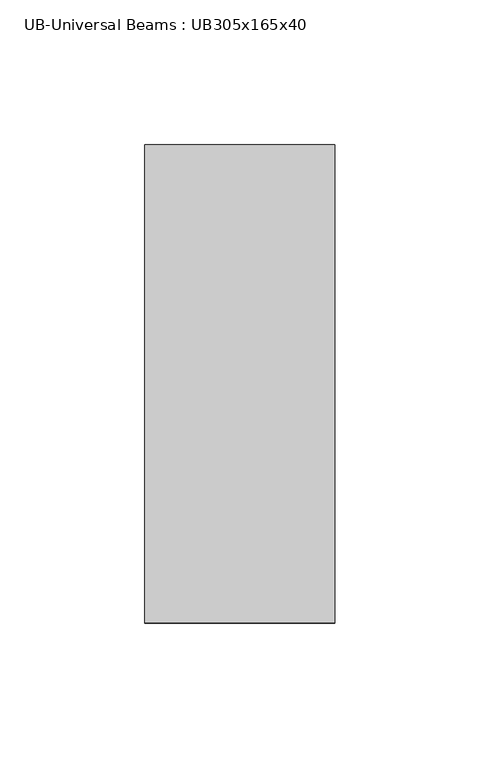
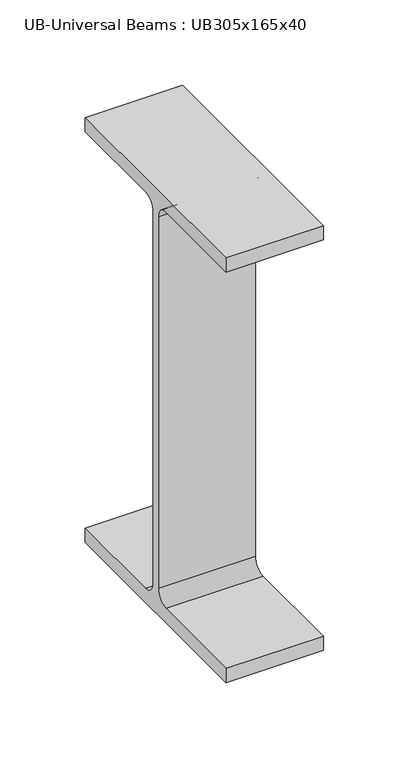
"""IFC4 building model written with IfcOpenShell, lengths in millimetres: beam geometry, UB-Universal Beams : UB305x165x40."""

from ifc_helpers import new_model, si_unit, point, frame, frame_2d, origin, place, context, project, spatial, polyline, circle_curve, trimmed, segment, composite_curve, outline, extrude, source, transform, mapped, element, save


def ub_universal_beams_ub305x165x40_454c3f6d(model_context):
    return source(origin(), model_context, "Body", "SweptSolid", [
        extrude(outline(composite_curve([segment(polyline([(82.5, -141.5), (82.5, -151.7), (-82.5, -151.7), (-82.5, -141.5), (-11.9, -141.5)]), True, "CONTINUOUS"), segment(trimmed(circle_curve(frame_2d((-11.9, -132.6)), 8.9), [point((-11.9, -141.5))], [point((-3.0, -132.6))], True, "CARTESIAN"), True, "CONTINUOUS"), segment(polyline([(-3.0, -132.6), (-3.0, 132.6)]), True, "CONTINUOUS"), segment(trimmed(circle_curve(frame_2d((-11.9, 132.6)), 8.9), [point((-3.0, 132.6))], [point((-11.9, 141.5))], True, "CARTESIAN"), True, "CONTINUOUS"), segment(polyline([(-11.9, 141.5), (-82.5, 141.5), (-82.5, 151.7), (82.5, 151.7), (82.5, 141.5), (11.9, 141.5)]), True, "CONTINUOUS"), segment(trimmed(circle_curve(frame_2d((11.9, 132.6)), 8.9), [point((11.9, 141.5))], [point((3.0, 132.6))], True, "CARTESIAN"), True, "CONTINUOUS"), segment(polyline([(3.0, 132.6), (3.0, -132.6)]), True, "CONTINUOUS"), segment(trimmed(circle_curve(frame_2d((11.9, -132.6)), 8.9), [point((3.0, -132.6))], [point((11.9, -141.5))], True, "CARTESIAN"), True, "CONTINUOUS"), segment(polyline([(11.9, -141.5), (82.5, -141.5)]), True, "CONTINUOUS")], self_intersect=False)), frame((-43.9, 0.0, 0.0), z_axis=(1.0, 0.0, 0.0), x_axis=(0.0, 1.0, 0.0)), (0.0, 0.0, 1.0), 65.6),
    ])


if __name__ == "__main__":
    model = new_model("IFC4")
    model_context = context("Model", 3, world=origin())
    ifc_project = project(units=[si_unit("LENGTHUNIT", "METRE", prefix="MILLI")], contexts=[model_context])
    site = spatial("IfcSite", under=ifc_project)
    building = spatial("IfcBuilding", under=site)
    placement = place(None, origin())
    ub_universal_beams_ub305x165x40_shape = ub_universal_beams_ub305x165x40_454c3f6d(model_context)
    element("IfcBeam", 1, ObjectType="UB-Universal Beams : UB305x165x40", at=placement, inside=building, context=model_context, shape_type="MappedRepresentation", body=[
        mapped(ub_universal_beams_ub305x165x40_shape, transform((0.0, 0.0, 0.0), x_axis=(1.0, 0.0, 0.0), y_axis=(0.0, 1.0, 0.0), z_axis=(0.0, 0.0, 1.0))),
    ])
    save(model, "model.ifc")

# Revit data of these elements
# Type "UB-Universal Beams : UB305x165x40"
#   Section Name Key = "UB305X165X40"
#   Width = 16.5 cm
#   Web Thickness = 0.6 cm
#   Web Fillet = 0.89 cm
#   Warping Constant = 164000.0 cm⁶
#   Torsional Moment of Inertia = 14.70 cm⁴
#   Section Area = 51.3 cm²
#   Plastic Modulus weak axis = 142.0 cm³
#   Plastic Modulus strong axis = 623.0 cm³
#   Nominal Weight = 40.2999 kgf/m
#   Moment of Inertia weak axis = 764.00 cm⁴
#   Moment of Inertia strong axis = 8503.00 cm⁴
#   Height = 30.34 cm
#   Flange Thickness = 1.02 cm
#   Elastic Modulus weak axis = 92.6 cm³
#   Elastic Modulus strong axis = 560.0 cm³
#   Centroid Vertical = 15.17 cm
#   Centroid Horizontal = 8.25 cm
#   Bolt Spacing = 9.0 cm
#   Length [instance default] = 1500 mm
#   Structural Material [instance default] = Metal - Steel 43-275
#   Type Comments = ""
#   Assembly Code = ""
# Element 1 (IfcBeam, "UB-Universal Beams : UB305x165x40")
#   Materials on its faces: "Metal - Steel 43-275"
# Materials
#   "Metal - Steel 43-275": class "Metal", colour RGB 247 247 247, transparency 0, Cost = 0
